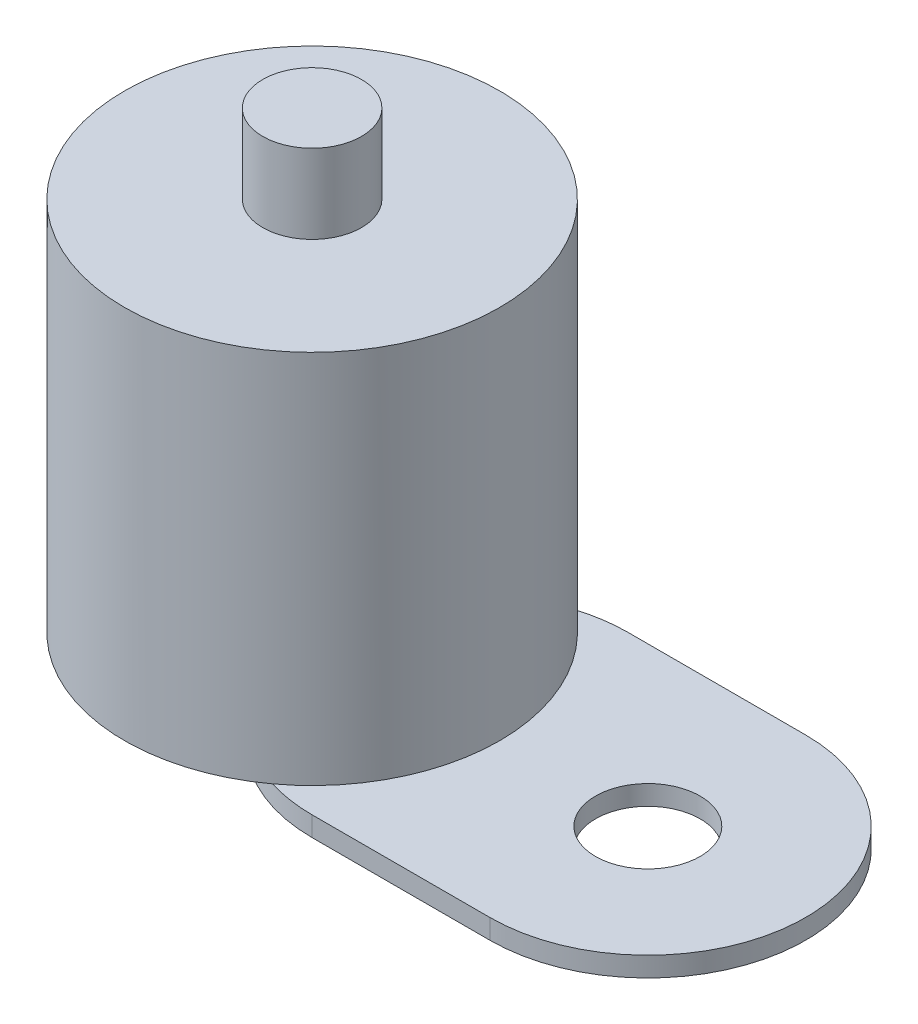
ISO-10303-21;
HEADER;
FILE_DESCRIPTION(('STEP AP214'),'2;1');
FILE_NAME('part.step','',(''),(''),'','','');
FILE_SCHEMA(('AUTOMOTIVE_DESIGN { 1 0 10303 214 1 1 1 1 }'));
ENDSEC;
DATA;
#1=APPLICATION_CONTEXT('core data for automotive mechanical design processes');
#2=APPLICATION_PROTOCOL_DEFINITION('international standard','automotive_design',2000,#1);
#3=PRODUCT_CONTEXT('',#1,'mechanical');
#4=PRODUCT('Part','Part','',(#3));
#5=PRODUCT_RELATED_PRODUCT_CATEGORY('part','',(#4));
#6=PRODUCT_DEFINITION_FORMATION('','',#4);
#7=PRODUCT_DEFINITION_CONTEXT('part definition',#1,'design');
#8=PRODUCT_DEFINITION('design','',#6,#7);
#9=PRODUCT_DEFINITION_SHAPE('','',#8);
#10=(LENGTH_UNIT() NAMED_UNIT(*) SI_UNIT(.MILLI.,.METRE.));
#11=(NAMED_UNIT(*) PLANE_ANGLE_UNIT() SI_UNIT($,.RADIAN.));
#12=(NAMED_UNIT(*) SI_UNIT($,.STERADIAN.) SOLID_ANGLE_UNIT());
#13=UNCERTAINTY_MEASURE_WITH_UNIT(LENGTH_MEASURE(1.E-05),#10,'distance_accuracy_value','');
#14=(GEOMETRIC_REPRESENTATION_CONTEXT(3) GLOBAL_UNCERTAINTY_ASSIGNED_CONTEXT((#13)) GLOBAL_UNIT_ASSIGNED_CONTEXT((#10,
#11,#12)) REPRESENTATION_CONTEXT('',''));
#15=CARTESIAN_POINT('',(0.,0.,0.));
#16=DIRECTION('',(0.,0.,1.));
#17=DIRECTION('',(1.,0.,0.));
#18=AXIS2_PLACEMENT_3D('',#15,#16,#17);
#19=CARTESIAN_POINT('',(-4.5,1.,0.));
#20=DIRECTION('',(0.,1.,0.));
#21=DIRECTION('',(0.,0.,1.));
#22=AXIS2_PLACEMENT_3D('',#19,#20,#21);
#23=PLANE('',#22);
#24=CARTESIAN_POINT('',(-12.5,1.,0.));
#25=DIRECTION('',(0.,1.,0.));
#26=DIRECTION('',(0.,0.,1.));
#27=AXIS2_PLACEMENT_3D('',#24,#25,#26);
#28=CIRCLE('',#27,9.5);
#29=CARTESIAN_POINT('',(-6.859375,1.,7.64417095631534));
#30=VERTEX_POINT('',#29);
#31=CARTESIAN_POINT('',(-6.859375,1.,-7.64417095631534));
#32=VERTEX_POINT('',#31);
#33=EDGE_CURVE('E54',#30,#32,#28,.T.);
#34=ORIENTED_EDGE('',*,*,#33,.F.);
#35=CARTESIAN_POINT('',(-4.5,1.,0.));
#36=DIRECTION('',(0.,1.,0.));
#37=DIRECTION('',(0.,0.,1.));
#38=AXIS2_PLACEMENT_3D('',#35,#36,#37);
#39=CIRCLE('',#38,8.);
#40=CARTESIAN_POINT('',(-4.5,1.,8.));
#41=VERTEX_POINT('',#40);
#42=EDGE_CURVE('E87',#30,#41,#39,.T.);
#43=ORIENTED_EDGE('',*,*,#42,.T.);
#44=DIRECTION('',(1.,0.,0.));
#45=VECTOR('',#44,1.);
#46=CARTESIAN_POINT('',(-4.5,1.,8.));
#47=LINE('',#46,#45);
#48=CARTESIAN_POINT('',(4.5,1.,8.));
#49=VERTEX_POINT('',#48);
#50=EDGE_CURVE('E92',#41,#49,#47,.T.);
#51=ORIENTED_EDGE('',*,*,#50,.T.);
#52=CARTESIAN_POINT('',(4.5,1.,0.));
#53=DIRECTION('',(0.,1.,0.));
#54=DIRECTION('',(0.,0.,1.));
#55=AXIS2_PLACEMENT_3D('',#52,#53,#54);
#56=CIRCLE('',#55,8.);
#57=CARTESIAN_POINT('',(4.5,1.,-8.));
#58=VERTEX_POINT('',#57);
#59=EDGE_CURVE('E125',#49,#58,#56,.T.);
#60=ORIENTED_EDGE('',*,*,#59,.T.);
#61=DIRECTION('',(-1.,0.,0.));
#62=VECTOR('',#61,1.);
#63=CARTESIAN_POINT('',(-4.5,1.,-8.));
#64=LINE('',#63,#62);
#65=CARTESIAN_POINT('',(-4.5,1.,-8.));
#66=VERTEX_POINT('',#65);
#67=EDGE_CURVE('E61',#58,#66,#64,.T.);
#68=ORIENTED_EDGE('',*,*,#67,.T.);
#69=EDGE_CURVE('E93',#66,#32,#39,.T.);
#70=ORIENTED_EDGE('',*,*,#69,.T.);
#71=EDGE_LOOP('',(#34,#43,#51,#60,#68,#70));
#72=FACE_BOUND('',#71,.T.);
#73=CARTESIAN_POINT('',(4.5,1.,0.));
#74=DIRECTION('',(0.,1.,0.));
#75=DIRECTION('',(0.,0.,1.));
#76=AXIS2_PLACEMENT_3D('',#73,#74,#75);
#77=CIRCLE('',#76,2.65);
#78=CARTESIAN_POINT('',(4.5,1.,2.65));
#79=VERTEX_POINT('',#78);
#80=EDGE_CURVE('E113',#79,#79,#77,.T.);
#81=ORIENTED_EDGE('',*,*,#80,.F.);
#82=EDGE_LOOP('',(#81));
#83=FACE_BOUND('',#82,.T.);
#84=ADVANCED_FACE('F39',(#72,#83),#23,.T.);
#85=CARTESIAN_POINT('',(-4.5,0.,0.));
#86=DIRECTION('',(0.,1.,0.));
#87=DIRECTION('',(0.,0.,1.));
#88=AXIS2_PLACEMENT_3D('',#85,#86,#87);
#89=PLANE('',#88);
#90=CARTESIAN_POINT('',(-4.5,0.,0.));
#91=DIRECTION('',(0.,1.,0.));
#92=DIRECTION('',(0.,0.,1.));
#93=AXIS2_PLACEMENT_3D('',#90,#91,#92);
#94=CIRCLE('',#93,8.);
#95=CARTESIAN_POINT('',(-4.5,0.,-8.));
#96=VERTEX_POINT('',#95);
#97=CARTESIAN_POINT('',(-4.5,0.,8.));
#98=VERTEX_POINT('',#97);
#99=EDGE_CURVE('E120',#96,#98,#94,.T.);
#100=ORIENTED_EDGE('',*,*,#99,.F.);
#101=DIRECTION('',(-1.,0.,0.));
#102=VECTOR('',#101,1.);
#103=CARTESIAN_POINT('',(-4.5,0.,-8.));
#104=LINE('',#103,#102);
#105=CARTESIAN_POINT('',(4.5,0.,-8.));
#106=VERTEX_POINT('',#105);
#107=EDGE_CURVE('E81',#106,#96,#104,.T.);
#108=ORIENTED_EDGE('',*,*,#107,.F.);
#109=CARTESIAN_POINT('',(4.5,0.,0.));
#110=DIRECTION('',(0.,1.,0.));
#111=DIRECTION('',(0.,0.,1.));
#112=AXIS2_PLACEMENT_3D('',#109,#110,#111);
#113=CIRCLE('',#112,8.);
#114=CARTESIAN_POINT('',(4.5,0.,8.));
#115=VERTEX_POINT('',#114);
#116=EDGE_CURVE('E129',#115,#106,#113,.T.);
#117=ORIENTED_EDGE('',*,*,#116,.F.);
#118=DIRECTION('',(1.,0.,0.));
#119=VECTOR('',#118,1.);
#120=CARTESIAN_POINT('',(-4.5,0.,8.));
#121=LINE('',#120,#119);
#122=EDGE_CURVE('E130',#98,#115,#121,.T.);
#123=ORIENTED_EDGE('',*,*,#122,.F.);
#124=EDGE_LOOP('',(#100,#108,#117,#123));
#125=FACE_BOUND('',#124,.T.);
#126=CARTESIAN_POINT('',(4.5,0.,0.));
#127=DIRECTION('',(0.,1.,0.));
#128=DIRECTION('',(0.,0.,1.));
#129=AXIS2_PLACEMENT_3D('',#126,#127,#128);
#130=CIRCLE('',#129,2.65);
#131=CARTESIAN_POINT('',(4.5,0.,2.65));
#132=VERTEX_POINT('',#131);
#133=EDGE_CURVE('E115',#132,#132,#130,.T.);
#134=ORIENTED_EDGE('',*,*,#133,.T.);
#135=EDGE_LOOP('',(#134));
#136=FACE_BOUND('',#135,.T.);
#137=ADVANCED_FACE('F144',(#125,#136),#89,.F.);
#138=CARTESIAN_POINT('',(-4.5,1.,0.));
#139=DIRECTION('',(0.,-1.,0.));
#140=DIRECTION('',(0.,0.,-1.));
#141=AXIS2_PLACEMENT_3D('',#138,#139,#140);
#142=CYLINDRICAL_SURFACE('',#141,8.);
#143=ORIENTED_EDGE('',*,*,#99,.T.);
#144=DIRECTION('',(0.,-1.,0.));
#145=VECTOR('',#144,1.);
#146=CARTESIAN_POINT('',(-4.5,1.,8.));
#147=LINE('',#146,#145);
#148=EDGE_CURVE('E43',#41,#98,#147,.T.);
#149=ORIENTED_EDGE('',*,*,#148,.F.);
#150=ORIENTED_EDGE('',*,*,#42,.F.);
#151=EDGE_CURVE('E96',#32,#30,#39,.T.);
#152=ORIENTED_EDGE('',*,*,#151,.F.);
#153=ORIENTED_EDGE('',*,*,#69,.F.);
#154=DIRECTION('',(0.,-1.,0.));
#155=VECTOR('',#154,1.);
#156=CARTESIAN_POINT('',(-4.5,1.,-8.));
#157=LINE('',#156,#155);
#158=EDGE_CURVE('E124',#66,#96,#157,.T.);
#159=ORIENTED_EDGE('',*,*,#158,.T.);
#160=EDGE_LOOP('',(#143,#149,#150,#152,#153,#159));
#161=FACE_BOUND('',#160,.T.);
#162=ADVANCED_FACE('F41',(#161),#142,.T.);
#163=CARTESIAN_POINT('',(-4.5,1.,8.));
#164=DIRECTION('',(0.,0.,-1.));
#165=DIRECTION('',(-1.,0.,0.));
#166=AXIS2_PLACEMENT_3D('',#163,#164,#165);
#167=PLANE('',#166);
#168=ORIENTED_EDGE('',*,*,#122,.T.);
#169=DIRECTION('',(0.,-1.,0.));
#170=VECTOR('',#169,1.);
#171=CARTESIAN_POINT('',(4.5,1.,8.));
#172=LINE('',#171,#170);
#173=EDGE_CURVE('E133',#49,#115,#172,.T.);
#174=ORIENTED_EDGE('',*,*,#173,.F.);
#175=ORIENTED_EDGE('',*,*,#50,.F.);
#176=ORIENTED_EDGE('',*,*,#148,.T.);
#177=EDGE_LOOP('',(#168,#174,#175,#176));
#178=FACE_BOUND('',#177,.T.);
#179=ADVANCED_FACE('F142',(#178),#167,.F.);
#180=CARTESIAN_POINT('',(4.5,1.,0.));
#181=DIRECTION('',(0.,-1.,0.));
#182=DIRECTION('',(0.,0.,-1.));
#183=AXIS2_PLACEMENT_3D('',#180,#181,#182);
#184=CYLINDRICAL_SURFACE('',#183,8.);
#185=ORIENTED_EDGE('',*,*,#116,.T.);
#186=DIRECTION('',(0.,-1.,0.));
#187=VECTOR('',#186,1.);
#188=CARTESIAN_POINT('',(4.5,1.,-8.));
#189=LINE('',#188,#187);
#190=EDGE_CURVE('E135',#58,#106,#189,.T.);
#191=ORIENTED_EDGE('',*,*,#190,.F.);
#192=ORIENTED_EDGE('',*,*,#59,.F.);
#193=ORIENTED_EDGE('',*,*,#173,.T.);
#194=EDGE_LOOP('',(#185,#191,#192,#193));
#195=FACE_BOUND('',#194,.T.);
#196=ADVANCED_FACE('F146',(#195),#184,.T.);
#197=CARTESIAN_POINT('',(-4.5,1.,-8.));
#198=DIRECTION('',(0.,0.,1.));
#199=DIRECTION('',(1.,0.,0.));
#200=AXIS2_PLACEMENT_3D('',#197,#198,#199);
#201=PLANE('',#200);
#202=ORIENTED_EDGE('',*,*,#107,.T.);
#203=ORIENTED_EDGE('',*,*,#158,.F.);
#204=ORIENTED_EDGE('',*,*,#67,.F.);
#205=ORIENTED_EDGE('',*,*,#190,.T.);
#206=EDGE_LOOP('',(#202,#203,#204,#205));
#207=FACE_BOUND('',#206,.T.);
#208=ADVANCED_FACE('F149',(#207),#201,.F.);
#209=CARTESIAN_POINT('',(4.5,1.,0.));
#210=DIRECTION('',(0.,-1.,0.));
#211=DIRECTION('',(0.,0.,-1.));
#212=AXIS2_PLACEMENT_3D('',#209,#210,#211);
#213=CYLINDRICAL_SURFACE('',#212,2.65);
#214=ORIENTED_EDGE('',*,*,#80,.T.);
#215=EDGE_LOOP('',(#214));
#216=FACE_BOUND('',#215,.T.);
#217=ORIENTED_EDGE('',*,*,#133,.F.);
#218=EDGE_LOOP('',(#217));
#219=FACE_BOUND('',#218,.T.);
#220=ADVANCED_FACE('F151',(#216,#219),#213,.F.);
#221=CARTESIAN_POINT('',(-12.5,1.,0.));
#222=DIRECTION('',(0.,1.,0.));
#223=DIRECTION('',(0.,0.,1.));
#224=AXIS2_PLACEMENT_3D('',#221,#222,#223);
#225=PLANE('',#224);
#226=EDGE_CURVE('E102',#32,#30,#28,.T.);
#227=ORIENTED_EDGE('',*,*,#226,.F.);
#228=ORIENTED_EDGE('',*,*,#151,.T.);
#229=EDGE_LOOP('',(#227,#228));
#230=FACE_BOUND('',#229,.T.);
#231=ADVANCED_FACE('F104',(#230),#225,.F.);
#232=CARTESIAN_POINT('',(-12.5,20.,0.));
#233=DIRECTION('',(0.,-1.,0.));
#234=DIRECTION('',(0.,0.,-1.));
#235=AXIS2_PLACEMENT_3D('',#232,#233,#234);
#236=CYLINDRICAL_SURFACE('',#235,9.5);
#237=CARTESIAN_POINT('',(-12.5,20.,0.));
#238=DIRECTION('',(0.,1.,0.));
#239=DIRECTION('',(0.,0.,1.));
#240=AXIS2_PLACEMENT_3D('',#237,#238,#239);
#241=CIRCLE('',#240,9.5);
#242=CARTESIAN_POINT('',(-12.5,20.,9.5));
#243=VERTEX_POINT('',#242);
#244=EDGE_CURVE('E109',#243,#243,#241,.T.);
#245=ORIENTED_EDGE('',*,*,#244,.F.);
#246=EDGE_LOOP('',(#245));
#247=FACE_BOUND('',#246,.T.);
#248=ORIENTED_EDGE('',*,*,#33,.T.);
#249=ORIENTED_EDGE('',*,*,#226,.T.);
#250=EDGE_LOOP('',(#248,#249));
#251=FACE_BOUND('',#250,.T.);
#252=ADVANCED_FACE('F108',(#247,#251),#236,.T.);
#253=CARTESIAN_POINT('',(-12.5,20.,0.));
#254=DIRECTION('',(0.,1.,0.));
#255=DIRECTION('',(0.,0.,1.));
#256=AXIS2_PLACEMENT_3D('',#253,#254,#255);
#257=PLANE('',#256);
#258=CARTESIAN_POINT('',(-12.5,20.,0.));
#259=DIRECTION('',(0.,1.,0.));
#260=DIRECTION('',(0.,0.,1.));
#261=AXIS2_PLACEMENT_3D('',#258,#259,#260);
#262=CIRCLE('',#261,2.5);
#263=CARTESIAN_POINT('',(-12.5,20.,2.5));
#264=VERTEX_POINT('',#263);
#265=EDGE_CURVE('E11',#264,#264,#262,.T.);
#266=ORIENTED_EDGE('',*,*,#265,.F.);
#267=EDGE_LOOP('',(#266));
#268=FACE_BOUND('',#267,.T.);
#269=ORIENTED_EDGE('',*,*,#244,.T.);
#270=EDGE_LOOP('',(#269));
#271=FACE_BOUND('',#270,.T.);
#272=ADVANCED_FACE('F168',(#268,#271),#257,.T.);
#273=CARTESIAN_POINT('',(-12.5,24.,0.));
#274=DIRECTION('',(0.,-1.,0.));
#275=DIRECTION('',(0.,0.,-1.));
#276=AXIS2_PLACEMENT_3D('',#273,#274,#275);
#277=CYLINDRICAL_SURFACE('',#276,2.5);
#278=CARTESIAN_POINT('',(-12.5,24.,0.));
#279=DIRECTION('',(0.,1.,0.));
#280=DIRECTION('',(0.,0.,1.));
#281=AXIS2_PLACEMENT_3D('',#278,#279,#280);
#282=CIRCLE('',#281,2.5);
#283=CARTESIAN_POINT('',(-12.5,24.,2.5));
#284=VERTEX_POINT('',#283);
#285=EDGE_CURVE('E110',#284,#284,#282,.T.);
#286=ORIENTED_EDGE('',*,*,#285,.F.);
#287=EDGE_LOOP('',(#286));
#288=FACE_BOUND('',#287,.T.);
#289=ORIENTED_EDGE('',*,*,#265,.T.);
#290=EDGE_LOOP('',(#289));
#291=FACE_BOUND('',#290,.T.);
#292=ADVANCED_FACE('F178',(#288,#291),#277,.T.);
#293=CARTESIAN_POINT('',(-12.5,24.,0.));
#294=DIRECTION('',(0.,1.,0.));
#295=DIRECTION('',(0.,0.,1.));
#296=AXIS2_PLACEMENT_3D('',#293,#294,#295);
#297=PLANE('',#296);
#298=ORIENTED_EDGE('',*,*,#285,.T.);
#299=EDGE_LOOP('',(#298));
#300=FACE_BOUND('',#299,.T.);
#301=ADVANCED_FACE('F179',(#300),#297,.T.);
#302=CLOSED_SHELL('',(#84,#137,#162,#179,#196,#208,#220,#231,#252,#272,#292,#301));
#303=MANIFOLD_SOLID_BREP('B2',#302);
#304=ADVANCED_BREP_SHAPE_REPRESENTATION('',(#18,#303),#14);
#305=SHAPE_DEFINITION_REPRESENTATION(#9,#304);
ENDSEC;
END-ISO-10303-21;
